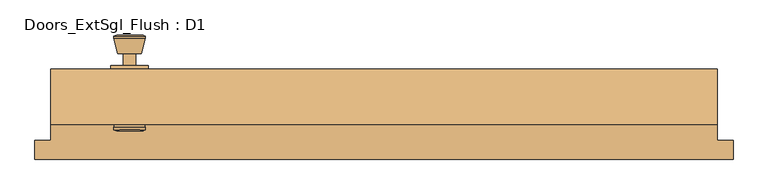
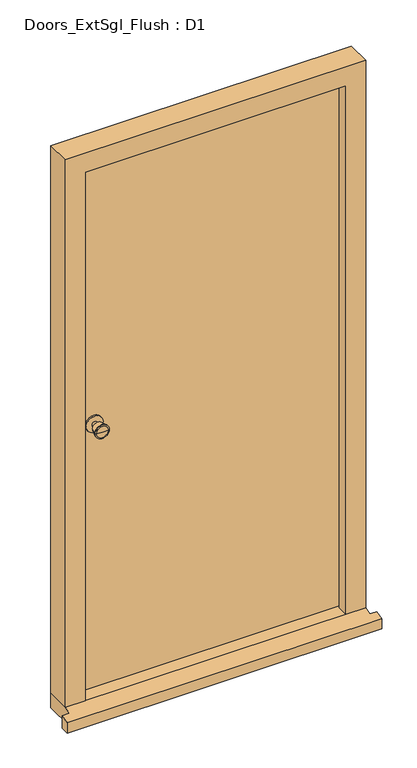
"""IFC4 building model written with IfcOpenShell, lengths in millimetres: door geometry, Doors_ExtSgl_Flush : D1."""

from ifc_helpers import new_model, si_unit, point, frame, frame_2d, origin, place, context, project, spatial, polyline, circle_curve, trimmed, segment, composite_curve, outline, extrude, faceted_brep, source, transform, mapped, element, save
from ifc_brep_helpers import plane_surface, cylinder_surface, revolved_surface, advanced_brep


def doors_extsgl_flush_d1_30a970b5(model_context):
    return source(origin(), model_context, "Body", "SolidModel", [
        advanced_brep(
        [(-406.9, 43.8, 1050.0), (-416.9, 43.8, 1050.0), (-396.9, 43.8, 1050.0), (-386.4241324, 92.8, 1050.0), (-427.3758676, 92.8, 1050.0), (-406.9, 92.8, 1050.0), (-381.9, 90.9721319, 1050.0), (-431.9, 90.9721319, 1050.0), (-381.9, 87.5084537, 1050.0), (-431.9, 87.5084537, 1050.0), (-388.263764, 62.8, 1050.0), (-425.536236, 62.8, 1050.0), (-396.9, 62.8, 1050.0), (-416.9, 62.8, 1050.0)],
        [
            (0, 1),
            (1, 2, circle_curve(frame((-406.9, 43.8, 1050.0), z_axis=(0.0, -1.0, 0.0), x_axis=(-1.0, 0.0, 0.0)), 10.0)),
            (2, 0),
            (2, 1, circle_curve(frame((-406.9, 43.8, 1050.0), z_axis=(0.0, -1.0, 0.0), x_axis=(-1.0, 0.0, 0.0)), 10.0)),
            (3, 4, circle_curve(frame((-406.9, 92.8, 1050.0), z_axis=(0.0, 1.0, 0.0), x_axis=(-1.0, 0.0, 0.0)), 20.4758676)),
            (4, 5),
            (5, 3),
            (4, 3, circle_curve(frame((-406.9, 92.8, 1050.0), z_axis=(0.0, 1.0, 0.0), x_axis=(-1.0, 0.0, 0.0)), 20.4758676)),
            (6, 7, circle_curve(frame((-406.9, 90.9721319, 1050.0), z_axis=(0.0, 1.0, 0.0), x_axis=(-1.0, 0.0, 0.0)), 25.0)),
            (7, 4),
            (3, 6),
            (7, 6, circle_curve(frame((-406.9, 90.9721319, 1050.0), z_axis=(0.0, 1.0, 0.0), x_axis=(-1.0, 0.0, 0.0)), 25.0)),
            (8, 9, circle_curve(frame((-406.9, 87.5084537, 1050.0), z_axis=(0.0, 1.0, 0.0), x_axis=(-1.0, 0.0, 0.0)), 25.0)),
            (9, 7),
            (6, 8),
            (9, 8, circle_curve(frame((-406.9, 87.5084537, 1050.0), z_axis=(0.0, 1.0, 0.0), x_axis=(-1.0, 0.0, 0.0)), 25.0)),
            (10, 11, circle_curve(frame((-406.9, 62.8, 1050.0), z_axis=(0.0, 1.0, 0.0), x_axis=(-1.0, 0.0, 0.0)), 18.636236)),
            (11, 9),
            (8, 10),
            (11, 10, circle_curve(frame((-406.9, 62.8, 1050.0), z_axis=(0.0, 1.0, 0.0), x_axis=(-1.0, 0.0, 0.0)), 18.636236)),
            (12, 13, circle_curve(frame((-406.9, 62.8, 1050.0), z_axis=(0.0, 1.0, 0.0), x_axis=(-1.0, 0.0, 0.0)), 10.0)),
            (13, 11),
            (10, 12),
            (13, 12, circle_curve(frame((-406.9, 62.8, 1050.0), z_axis=(0.0, 1.0, 0.0), x_axis=(-1.0, 0.0, 0.0)), 10.0)),
            (1, 13),
            (12, 2),
        ],
        [
            plane_surface(frame((-406.9, 43.8, 1050.0), z_axis=(0.0, -1.0, 0.0), x_axis=(-1.0, 0.0, 0.0))),
            plane_surface(frame((-406.9, 92.8, 1050.0), z_axis=(0.0, 1.0, 0.0), x_axis=(-1.0, 0.0, 0.0))),
            revolved_surface(polyline([(-427.3758676, 92.8, 1050.0), (-431.9, 90.9721319, 1050.0)]), (-406.9, 43.8, 1050.0), (0.0, -1.0, 0.0)),
            cylinder_surface(frame((-406.9, 43.8, 1050.0), z_axis=(0.0, -1.0, 0.0), x_axis=(-1.0, 0.0, 0.0)), 25.0),
            revolved_surface(polyline([(-431.9, 87.5084537, 1050.0), (-425.536236, 62.8, 1050.0)]), (-406.9, 43.8, 1050.0), (0.0, -1.0, 0.0)),
            plane_surface(frame((-406.9, 62.8, 1050.0), z_axis=(0.0, -1.0, 0.0), x_axis=(-1.0, 0.0, 0.0))),
            cylinder_surface(frame((-406.9, 43.8, 1050.0), z_axis=(0.0, -1.0, 0.0), x_axis=(-1.0, 0.0, 0.0)), 10.0),
        ],
        [
            (0, [[1, 2, 3]]),
            (0, [[-3, 4, -1]]),
            (1, [[5, 6, 7]]),
            (1, [[8, -7, -6]]),
            (2, [[9, 10, -5, 11]]),
            (2, [[12, -11, -8, -10]]),
            (3, [[13, 14, -9, 15]]),
            (3, [[16, -15, -12, -14]]),
            (4, [[17, 18, -13, 19]]),
            (4, [[20, -19, -16, -18]]),
            (5, [[21, 22, -17, 23]]),
            (5, [[24, -23, -20, -22]]),
            (6, [[-2, 25, -21, 26]]),
            (6, [[-4, -26, -24, -25]]),
        ],
    ),
        extrude(outline(composite_curve([segment(trimmed(circle_curve(frame_2d((1050.0, -406.9)), 30.0), [point((1050.0, -436.9))], [point((1050.0, -376.9))], False, "CARTESIAN"), True, "CONTINUOUS"), segment(trimmed(circle_curve(frame_2d((1050.0, -406.9)), 30.0), [point((1050.0, -376.9))], [point((1050.0, -436.9))], False, "CARTESIAN"), True, "CONTINUOUS")], self_intersect=False)), frame((0.0, 37.8, 0.0), z_axis=(0.0, 1.0, 0.0), x_axis=(0.0, 0.0, 1.0)), (0.0, 0.0, 1.0), 6.0),
        advanced_brep(
        [(-406.9, -12.2, 1050.0), (-396.9, -12.2, 1050.0), (-416.9, -12.2, 1050.0), (-386.4241324, -61.2, 1050.0), (-406.9, -61.2, 1050.0), (-427.3758676, -61.2, 1050.0), (-381.9, -59.3721319, 1050.0), (-431.9, -59.3721319, 1050.0), (-381.9, -55.9084537, 1050.0), (-431.9, -55.9084537, 1050.0), (-388.263764, -31.2, 1050.0), (-425.536236, -31.2, 1050.0), (-396.9, -31.2, 1050.0), (-416.9, -31.2, 1050.0)],
        [
            (0, 1),
            (1, 2, circle_curve(frame((-406.9, -12.2, 1050.0), z_axis=(0.0, 1.0, 0.0), x_axis=(-1.0, 0.0, 0.0)), 10.0)),
            (2, 0),
            (2, 1, circle_curve(frame((-406.9, -12.2, 1050.0), z_axis=(0.0, 1.0, 0.0), x_axis=(-1.0, 0.0, 0.0)), 10.0)),
            (3, 4),
            (4, 5),
            (5, 3, circle_curve(frame((-406.9, -61.2, 1050.0), z_axis=(0.0, -1.0, 0.0), x_axis=(-1.0, 0.0, 0.0)), 20.4758676)),
            (3, 5, circle_curve(frame((-406.9, -61.2, 1050.0), z_axis=(0.0, -1.0, 0.0), x_axis=(-1.0, 0.0, 0.0)), 20.4758676)),
            (6, 3),
            (5, 7),
            (7, 6, circle_curve(frame((-406.9, -59.3721319, 1050.0), z_axis=(0.0, -1.0, 0.0), x_axis=(-1.0, 0.0, 0.0)), 25.0)),
            (6, 7, circle_curve(frame((-406.9, -59.3721319, 1050.0), z_axis=(0.0, -1.0, 0.0), x_axis=(-1.0, 0.0, 0.0)), 25.0)),
            (8, 6),
            (7, 9),
            (9, 8, circle_curve(frame((-406.9, -55.9084537, 1050.0), z_axis=(0.0, -1.0, 0.0), x_axis=(-1.0, 0.0, 0.0)), 25.0)),
            (8, 9, circle_curve(frame((-406.9, -55.9084537, 1050.0), z_axis=(0.0, -1.0, 0.0), x_axis=(-1.0, 0.0, 0.0)), 25.0)),
            (10, 8),
            (9, 11),
            (11, 10, circle_curve(frame((-406.9, -31.2, 1050.0), z_axis=(0.0, -1.0, 0.0), x_axis=(-1.0, 0.0, 0.0)), 18.636236)),
            (10, 11, circle_curve(frame((-406.9, -31.2, 1050.0), z_axis=(0.0, -1.0, 0.0), x_axis=(-1.0, 0.0, 0.0)), 18.636236)),
            (12, 10),
            (11, 13),
            (13, 12, circle_curve(frame((-406.9, -31.2, 1050.0), z_axis=(0.0, -1.0, 0.0), x_axis=(-1.0, 0.0, 0.0)), 10.0)),
            (12, 13, circle_curve(frame((-406.9, -31.2, 1050.0), z_axis=(0.0, -1.0, 0.0), x_axis=(-1.0, 0.0, 0.0)), 10.0)),
            (1, 12),
            (13, 2),
        ],
        [
            plane_surface(frame((-406.9, -12.2, 1050.0), z_axis=(0.0, 1.0, 0.0), x_axis=(-1.0, 0.0, 0.0))),
            plane_surface(frame((-406.9, -61.2, 1050.0), z_axis=(0.0, -1.0, 0.0), x_axis=(-1.0, 0.0, 0.0))),
            revolved_surface(polyline([(-427.3758676, -61.2, 1050.0), (-431.9, -59.3721319, 1050.0)]), (-406.9, -12.2, 1050.0), (0.0, 1.0, 0.0)),
            cylinder_surface(frame((-406.9, -12.2, 1050.0), z_axis=(0.0, 1.0, 0.0), x_axis=(-1.0, 0.0, 0.0)), 25.0),
            revolved_surface(polyline([(-431.9, -55.9084537, 1050.0), (-425.536236, -31.2, 1050.0)]), (-406.9, -12.2, 1050.0), (0.0, 1.0, 0.0)),
            plane_surface(frame((-406.9, -31.2, 1050.0), z_axis=(0.0, 1.0, 0.0), x_axis=(-1.0, 0.0, 0.0))),
            cylinder_surface(frame((-406.9, -12.2, 1050.0), z_axis=(0.0, 1.0, 0.0), x_axis=(-1.0, 0.0, 0.0)), 10.0),
        ],
        [
            (0, [[1, 2, 3]]),
            (0, [[-3, 4, -1]]),
            (1, [[5, 6, 7]]),
            (1, [[-6, -5, 8]]),
            (2, [[9, -7, 10, 11]]),
            (2, [[-10, -8, -9, 12]]),
            (3, [[13, -11, 14, 15]]),
            (3, [[-14, -12, -13, 16]]),
            (4, [[17, -15, 18, 19]]),
            (4, [[-18, -16, -17, 20]]),
            (5, [[21, -19, 22, 23]]),
            (5, [[-22, -20, -21, 24]]),
            (6, [[25, -23, 26, -2]]),
            (6, [[-26, -24, -25, -4]]),
        ],
    ),
        extrude(outline(composite_curve([segment(trimmed(circle_curve(frame_2d((1050.0, -406.9)), 30.0), [point((1050.0, -436.9))], [point((1050.0, -376.9))], False, "CARTESIAN"), True, "CONTINUOUS"), segment(trimmed(circle_curve(frame_2d((1050.0, -406.9)), 30.0), [point((1050.0, -376.9))], [point((1050.0, -436.9))], False, "CARTESIAN"), True, "CONTINUOUS")], self_intersect=False)), frame((0.0, -12.2, 0.0), z_axis=(0.0, 1.0, 0.0), x_axis=(0.0, 0.0, 1.0)), (0.0, 0.0, 1.0), 6.0),
        faceted_brep([(462.9, -51.2, 54.5), (462.9, -9.2, 54.5), (484.9, -9.2, 54.5), (484.9, 37.8, 54.5), (533.4, 37.8, 54.5), (533.4, -51.2, 54.5), (533.4, -51.2, 2110.0), (-533.4, -51.2, 2110.0), (-533.4, -51.2, 54.5), (-462.9, -51.2, 54.5), (-462.9, -51.2, 2039.5), (462.9, -51.2, 2039.5), (533.4, 37.8, 2110.0), (484.9, 37.8, 2061.5), (-484.9, 37.8, 2061.5), (-484.9, 37.8, 54.5), (-533.4, 37.8, 54.5), (-533.4, 37.8, 2110.0), (484.9, -9.2, 2061.5), (462.9, -9.2, 2039.5), (-462.9, -9.2, 2039.5), (-462.9, -9.2, 54.5), (-484.9, -9.2, 54.5), (-484.9, -9.2, 2061.5)], [[[0, 1, 2, 3, 4, 5]], [[5, 6, 7, 8, 9, 10, 11, 0]], [[4, 12, 6, 5]], [[3, 13, 14, 15, 16, 17, 12, 4]], [[2, 18, 13, 3]], [[1, 19, 20, 21, 22, 23, 18, 2]], [[0, 11, 19, 1]], [[10, 9, 21, 20]], [[9, 8, 16, 15, 22, 21]], [[17, 16, 8, 7]], [[23, 22, 15, 14]], [[12, 17, 7, 6]], [[18, 23, 14, 13]], [[11, 10, 20, 19]]]),
        extrude(outline(polyline([(481.9, 37.8), (481.9, -6.2), (-482.8250294, -6.2), (-482.8250294, 37.8), (481.9, 37.8)])), frame((0.0, 0.0, 58.5), z_axis=(0.0, 0.0, 1.0), x_axis=(1.0, 0.0, 0.0)), (0.0, 0.0, 1.0), 2000.0),
        faceted_brep([(558.4, -106.2, 0.0), (558.4, -76.2, 0.0), (558.4, -76.2, 47.2703282), (558.4, -106.2, 38.5947221), (-558.4, -106.2, 38.5947221), (-558.4, -76.2, 47.2703282), (-558.4, -76.2, 0.0), (-558.4, -106.2, 0.0), (-533.4, -76.2, 0.0), (-533.4, 37.8, 0.0), (533.4, 37.8, 0.0), (533.4, -76.2, 0.0), (533.4, -76.2, 47.2703282), (533.4, -51.2, 54.5), (-533.4, -51.2, 54.5), (-533.4, -76.2, 47.2703282), (533.4, 37.8, 54.5), (-533.4, 37.8, 54.5)], [[[0, 1, 2, 3]], [[4, 5, 6, 7]], [[7, 6, 8, 9, 10, 11, 1, 0]], [[3, 4, 7, 0]], [[3, 2, 12, 13, 14, 15, 5, 4]], [[14, 13, 16, 17]], [[17, 16, 10, 9]], [[15, 14, 17, 9, 8]], [[8, 6, 5, 15]], [[11, 10, 16, 13, 12]], [[12, 2, 1, 11]]]),
    ])


if __name__ == "__main__":
    model = new_model("IFC4")
    model_context = context("Model", 3, world=origin())
    ifc_project = project(units=[si_unit("LENGTHUNIT", "METRE", prefix="MILLI")], contexts=[model_context])
    site = spatial("IfcSite", under=ifc_project)
    building = spatial("IfcBuilding", under=site)
    placement = place(None, origin())
    doors_extsgl_flush_d1_shape = doors_extsgl_flush_d1_30a970b5(model_context)
    element("IfcDoor", 1, ObjectType="Doors_ExtSgl_Flush : D1", at=placement, inside=building, context=model_context, shape_type="MappedRepresentation", body=[
        mapped(doors_extsgl_flush_d1_shape, transform((0.0, 0.0, 0.0), x_axis=(1.0, 0.0, 0.0), y_axis=(0.0, 1.0, 0.0), z_axis=(0.0, 0.0, 1.0))),
    ])
    save(model, "model.ifc")

# Revit data of these elements
# Type "Doors_ExtSgl_Flush : D1"
#   Type Mark = "49"
#   Type Comments = "External Single"
#   Operation = "SingleSwingRight"
#   Construction Type Id = "MDOOR"
#   Keynote = "L20"
#   Analytic Construction = "Metal"
#   Wrap Layers (Int) from Ext = 177.5 mm
#   Wrap Layers (Ext) from Ext = 102.5 mm
#   Thickness = 44 mm
#   Rough Width = 1066.8 mm
#   Rough Height = 2110 mm
#   O/A Frame Width = 64 mm
#   Heat Transfer Coefficient (U) = 3.7021 W/(m²·K)
#   Handle Z Distance = 1050 mm
#   FrameWidth = 42 mm
#   FrameOffset - External = 25 mm
#   FrameDepth = 89 mm
#   Door Panel Width = 963.8 mm
#   Door Panel Thickness = 44 mm
#   Door Panel Height = 2000 mm
#   Cill Thickness = 54.5 mm
#   Cill Projection = 30 mm
#   Handle X Distance = 75 mm
#   Height = 2110 mm
#   Structural Tolerance = 6.5 mm
#   Tolerance = 3 mm
#   Undercut = 4 mm
#   Width = 1066.8 mm
#   Cill Extension = 25 mm
#   Cavity Closer Width = 50 mm
#   Cavity Closer Offset from Ext = 102.5 mm
#   Cavity Closer Depth = 85 mm
#   Vis - Ironmongery = yes
#   Vis - Cavity Closers = yes
#   Define Thermal Properties by = 1
#   Function = 1
#   Material Door = Door - Panel
#   Material Frame = Door - Frame/Mullion
#   Material Ironmongery = Door - Handle
#   Visual Light Transmittance = 0
#   Solar Heat Gain Coefficient = 0
#   Wall Closure = (empty or 0)
# Element 1 (IfcDoor, "Doors_ExtSgl_Flush : D1")
#   Materials on its faces: "Door - Handle", "Door - Frame/Mullion", "Door - Panel"
# Materials
#   "Door - Panel": class "Wood", colour RGB 210 159 95, transparency 0, Keynote = "L20", Cost = 0
#   "Door - Frame/Mullion": class "Wood", colour RGB 212 179 113, transparency 0, Keynote = "L20", Cost = 0
#   "Door - Handle": colour RGB 0 0 0, transparency 0, Keynote = "P21", Cost = 0
